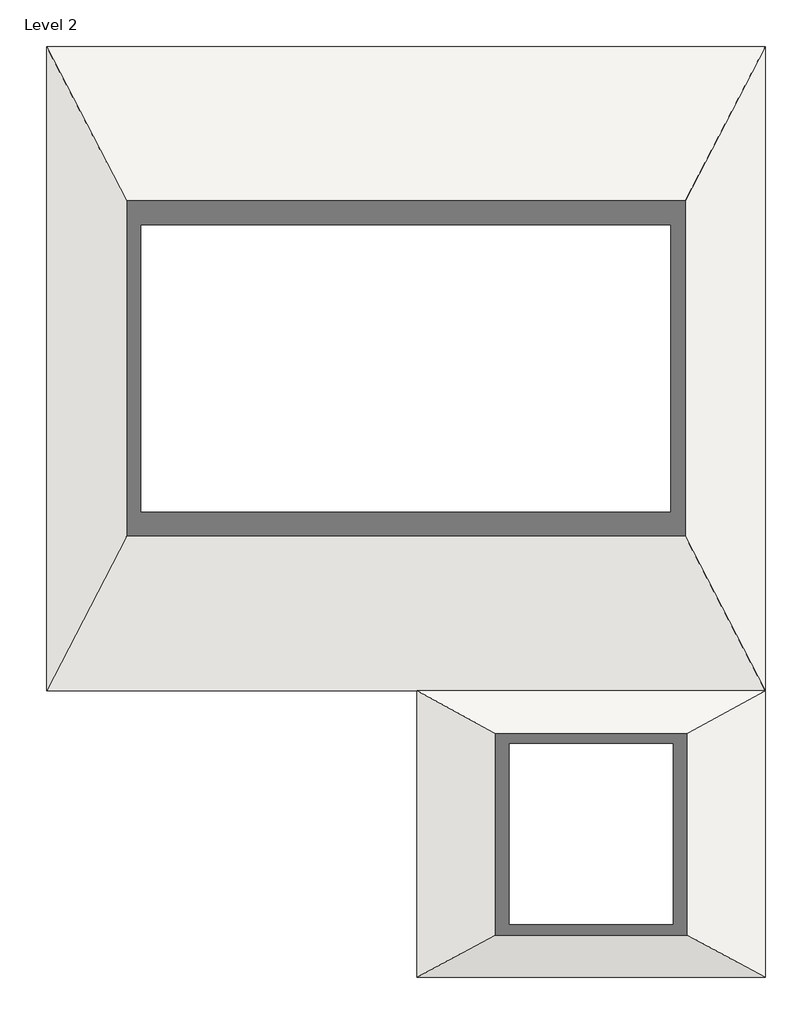
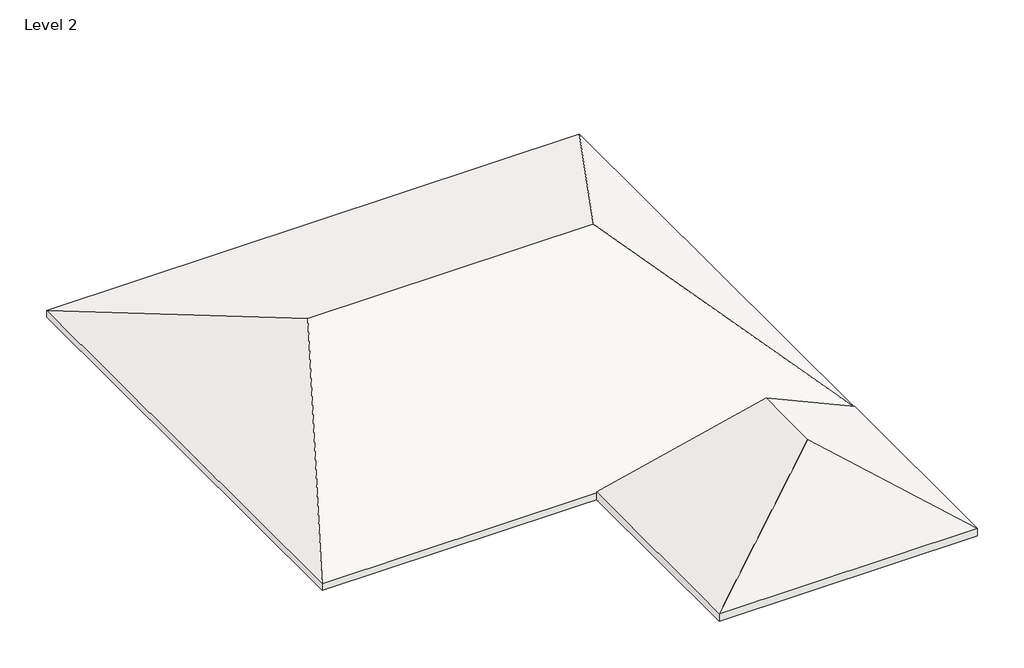
# One storey: 2 roofs.
"""IFC4 building model written with IfcOpenShell, lengths in millimetres."""

from ifc_helpers import new_model, si_unit, origin, place, context, project, spatial, faceted_brep, element, save

model = new_model("IFC4")

# Units and contexts
model_context = context("Model", 3, world=origin())
ifc_project = project(units=[si_unit("LENGTHUNIT", "METRE", prefix="MILLI")], contexts=[model_context])

# Site, building, storey
site = spatial("IfcSite", under=ifc_project)
building = spatial("IfcBuilding", under=site)
storey = spatial("IfcBuildingStorey", under=building, Name="Level 2", Elevation=3048.0)

# Roofs
placement = place(None, origin())
element("IfcRoof", 1, ObjectType="6\"", at=placement, inside=storey, context=model_context, shape_type="Brep", body=[
    faceted_brep([(-633.8367641, 9060.9670221, 3048.0), (-3515.6735642, 3498.3670221, 5209.3776001), (-10100.6001588, 3498.3670221, 5209.3776001), (-12982.4369589, 9060.9670221, 3048.0), (-12982.4369589, -2064.2329779, 3048.0), (-633.8367641, -2064.2329779, 3048.0), (-597.8368615, 9060.9670221, 3211.5000731), (-13018.4368615, 9060.9670221, 3211.5000731), (-10136.6000614, 3498.3670221, 5372.8776731), (-3479.6736616, 3498.3670221, 5372.8776731), (-13018.4368615, -2064.2329779, 3211.5000731), (-597.8368615, -2064.2329779, 3211.5000731), (-13018.4368615, 9060.9670221, 3048.0), (-597.8368615, 9060.9670221, 3048.0), (-13018.4368615, -2064.2329779, 3048.0), (-597.8368615, -2064.2329779, 3048.0)], [[[0, 1, 2, 3]], [[3, 2, 4]], [[4, 2, 1, 5]], [[1, 0, 5]], [[6, 7, 8, 9]], [[7, 10, 8]], [[10, 11, 9, 8]], [[6, 9, 11]], [[12, 7, 6, 13, 0, 3]], [[14, 10, 7, 12]], [[15, 11, 10, 14, 4, 5]], [[13, 6, 11, 15]], [[13, 15, 5, 0]], [[4, 14, 12, 3]]]),
])
element("IfcRoof", 2, ObjectType="6\"", at=placement, inside=storey, context=model_context, shape_type="Brep", body=[
    faceted_brep([(-597.8368615, -2114.3477098, 3048.0), (-3607.7368615, -3751.2365701, 5305.425), (-6617.6368615, -2114.3477098, 3048.0), (-3607.7368615, -5330.2293856, 5305.425), (-6617.6368615, -6967.118246, 3048.0), (-597.8368615, -6967.118246, 3048.0), (-597.8368615, -2064.2329779, 3238.5), (-6617.6368615, -2064.2329779, 3238.5), (-3607.7368615, -3701.1218382, 5495.925), (-6617.6368615, -7017.2329779, 3238.5), (-3607.7368615, -5380.3441176, 5495.925), (-597.8368615, -7017.2329779, 3238.5), (-6617.6368615, -2064.2329779, 3048.0), (-597.8368615, -2064.2329779, 3048.0), (-6617.6368615, -7017.2329779, 3048.0), (-597.8368615, -7017.2329779, 3048.0)], [[[0, 1, 2]], [[2, 1, 3, 4]], [[4, 3, 5]], [[1, 0, 5, 3]], [[6, 7, 8]], [[7, 9, 10, 8]], [[9, 11, 10]], [[6, 8, 10, 11]], [[12, 7, 6, 13]], [[14, 9, 7, 12, 2, 4]], [[15, 11, 9, 14]], [[13, 6, 11, 15, 5, 0]], [[13, 0, 2, 12]], [[5, 15, 14, 4]]]),
])

save(model, "model.ifc")

# Revit data of these elements
# Type "6\""
#   Assembly Code = "B1020"
#   Layers, outside or top first: 0' - 6" "ROOF" (function 1)
# Element 1 (IfcRoof, "6\"")
#   built-in parameter 1001705 = 17.6276 (stored number, unit not read)
#   built-in parameter 1001710 = 33615
#   Phase Created = New Construction
#   Materials on its faces: "ROOF"
# Element 2 (IfcRoof, "6\"")
#   built-in parameter 1001705 = 18.0312 (stored number, unit not read)
#   built-in parameter 1001710 = 33615
#   Phase Created = New Construction
#   Materials on its faces: "ROOF"
# Materials
#   "ROOF": class "Generic", colour RGB 64 86 97, transparency 0, Cost = 0
